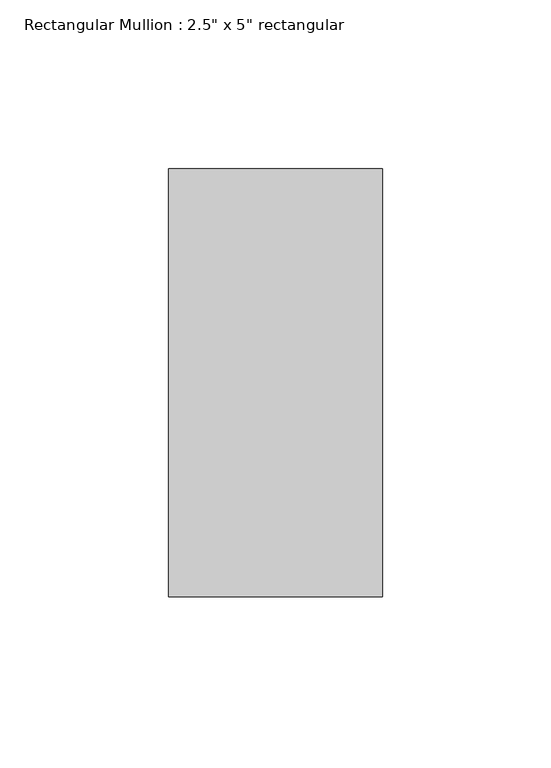
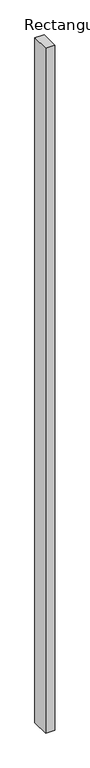
"""IFC4 building model written with IfcOpenShell, lengths in millimetres: member geometry."""

from ifc_helpers import new_model, si_unit, frame, origin, place, context, project, spatial, polyline, outline, extrude, source, transform, mapped, element, save


def member_cd715f5c(model_context):
    return source(origin(), model_context, "Body", "SweptSolid", [
        extrude(outline(polyline([(0.0, 63.5), (0.0, -63.5), (-63.5, -63.5), (-63.5, 63.5), (0.0, 63.5)])), frame((0.0, 0.0, -5003.8), z_axis=(0.0, 0.0, 1.0), x_axis=(1.0, 0.0, 0.0)), (0.0, 0.0, 1.0), 5003.8),
    ])


if __name__ == "__main__":
    model = new_model("IFC4")
    model_context = context("Model", 3, world=origin())
    ifc_project = project(units=[si_unit("LENGTHUNIT", "METRE", prefix="MILLI")], contexts=[model_context])
    site = spatial("IfcSite", under=ifc_project)
    building = spatial("IfcBuilding", under=site)
    placement = place(None, origin())
    member_shape = member_cd715f5c(model_context)
    element("IfcMember", 1, ObjectType="Rectangular Mullion : 2.5\" x 5\" rectangular", at=placement, inside=building, context=model_context, shape_type="MappedRepresentation", body=[
        mapped(member_shape, transform((0.0, 0.0, 0.0), x_axis=(1.0, 0.0, 0.0), y_axis=(0.0, 1.0, 0.0), z_axis=(0.0, 0.0, 1.0))),
    ])
    save(model, "model.ifc")

# Revit data of these elements
# Type "Rectangular Mullion : 2.5\" x 5\" rectangular"
#   built-in parameter 1007304 = 0.416667 (stored number, unit not read)
#   built-in parameter 1007301 = 0.104167 (stored number, unit not read)
#   built-in parameter 1007300 = 0.104167 (stored number, unit not read)
# Element 1 (IfcMember, "Rectangular Mullion : 2.5\" x 5\" rectangular")
#   Materials on its faces: "Iron, Ductile"
# Materials
#   "Iron, Ductile": class "Metal", colour RGB 0 0 0, transparency 0, Description = "Ductile cast iron", Cost = 0
